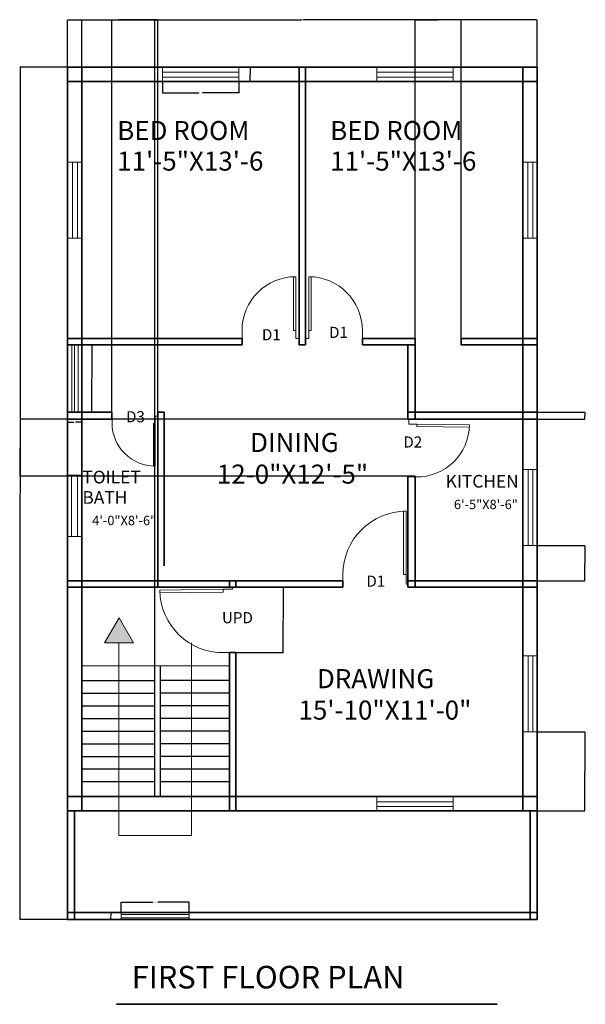
# Model space of a CAD drawing. Units: inches. Extents: x 2000 to 5103, y 1720 to 4295.
# Tile 2 of 2: x 2539 to 2895, y 1750 to 2371. Entities that reach past the tile are written whole.
import ezdxf

# ---------------------------------------------------------------- set-up
doc = ezdxf.new("R2010")
doc.units = ezdxf.units.IN
for name, color, linetype, lineweight in [('A-ANNO-DIMS', 2, 'Continuous', 18), ('A-ANNO-SYMB', 7, 'Continuous', 18), ('A-ANNO-TEXT', 3, 'Continuous', 18), ('A-ANNO-TITL', 7, 'Continuous', 35), ('A-AREA-IDEN', 7, 'Continuous', 25), ('A-DOOR', 4, 'Continuous', 18), ('A-WALL', 7, 'Continuous', 35), ('stair', 7, 'Continuous', 25), ('window', 10, 'Continuous', 18)]:
    doc.layers.add(name, color=color, linetype=linetype, lineweight=lineweight)
doc.styles.get("Standard").update_dxf_attribs({"font": 'arial.ttf'})
doc.dimstyles.get("Standard").update_dxf_attribs({"dimtxt": 0.18, "dimasz": 0.18, "dimexe": 0.18, "dimexo": 0.0625, "dimgap": 0.09, "dimtad": 0, "dimtih": 1, "dimtoh": 1, "dimdec": 4, "dimzin": 0, "dimdsep": 46, "dimtxsty": 'Standard', "dimcen": 0.09, "dimadec": 0, "dimazin": 0, "dimtfac": 1, "dimtdec": 4, "dimtofl": 0, "dimtmove": 0, "dimatfit": 3, "dimfxl": 1, "dimtolj": 1, "dimtzin": 0, "dimarcsym": 0})

# ---------------------------------------------------------------- blocks, each defined once
blk = doc.blocks.new('Dining Set - 36 x 72 in')
at = {"layer": 'window'}
for p, q in [((418.4, 887.02), (466.4, 887.02)), ((418.4, 883.92), (466.4, 883.92))]:
    blk.add_line(p, q, dxfattribs=at)
blk.add_lwpolyline([(418.4, 881.14), (418.4, 890.14), (466.4, 890.14), (466.4, 881.14)], close=True, dxfattribs=at)
blk = doc.blocks.new('*U3')
for p, q in [((0, 0), (0, -6)), ((40, 0), (40, -6))]:
    blk.add_line(p, q)
blk.add_lwpolyline([(0, 0), (0, 40), (1.75, 40), (1.75, 0)], close=True)
blk.add_arc((0, 0), 40, 0, 90)
blk = doc.blocks.new('WIN-DINING')
for p, q in [((2.68, 42.5), (2.68, 0)), ((4.5, 42.5), (4.5, 0)), ((6.78, 42.5), (6.78, 0))]:
    blk.add_line(p, q)
blk.add_lwpolyline([(0, 42.5), (9, 42.5), (9, 0), (0, 0)], close=True)
blk = doc.blocks.new('WIN-BATH')
for p, q in [((2.49, 38.59), (2.49, 0)), ((6.38, 38.59), (6.38, 0)), ((6.38, 38.59), (6.38, 0))]:
    blk.add_line(p, q)
blk.add_lwpolyline([(0, 38.59), (9, 38.59), (9, 0), (0, 0)], close=True)
blk = doc.blocks.new('WIN-FRONT')
for p, q in [((0, 3.25), (43.02, 3.25)), ((0, 1.25), (43.02, 1.25))]:
    blk.add_line(p, q)
blk.add_lwpolyline([(0, 4.5), (43.02, 4.5), (43.02, 0), (0, 0)], close=True)
blk = doc.blocks.new('STAIR-RETURN-FLIGHTS')
for p, q in [((93.06, 82.39), (0, 82.3)), ((46.1, 0), (46.1, 82.34)), ((49.5, 82.35), (49.5, 0)), ((0, 73.28), (46.1, 73.28)), ((49.5, 73.48), (93.06, 73.48)), ((0, 65.3), (46.1, 65.3)), ((49.5, 65.5), (93.06, 65.5)), ((0, 57.32), (46.1, 57.32)), ((49.5, 57.52), (93.06, 57.52)), ((0, 49.34), (46.1, 49.34)), ((49.5, 49.54), (93.06, 49.54)), ((0, 41.37), (46.1, 41.37)), ((49.5, 41.56), (93.06, 41.56)), ((0, 33.39), (46.1, 33.39)), ((49.5, 33.58), (93.06, 33.58)), ((0, 25.41), (46.1, 25.41)), ((49.5, 25.61), (93.06, 25.61)), ((0, 17.43), (46.1, 17.43)), ((49.5, 17.63), (93.06, 17.63)), ((0, 9.45), (46.1, 9.45)), ((49.5, 9.65), (93.06, 9.65))]:
    blk.add_line(p, q)
blk = doc.blocks.new('STAIR-PATH-ARROW')
h = blk.add_hatch(color=256)
h.dxf.hatch_style = 1
h.paths.add_polyline_path([(9.07, 137.14), (0, 121.43), (18.13, 121.43)])
for p, q in [((0, 121.43), (9.07, 137.14)), ((9.07, 137.14), (18.13, 121.43)), ((18.13, 121.43), (0, 121.43)), ((8.84, 0), (8.84, 121.43)), ((8.84, 121.43), (18.13, 121.43)), ((54.71, 121.43), (54.71, 0)), ((54.71, 0), (8.84, 0))]:
    blk.add_line(p, q)
blk = doc.blocks.new('*D9')
at = {"layer": 'A-ANNO-DIMS', "color": 0, "lineweight": -2, "transparency": 16777216}
for p, q in [((2629.1, 2331.91), (2629.1, 2324.59)), ((2677.1, 2331.91), (2677.1, 2324.59)), ((2629.28, 2324.77), (2651.98, 2324.77)), ((2676.92, 2324.77), (2654.22, 2324.77))]:
    blk.add_line(p, q, dxfattribs=at)
at = {"layer": 'A-ANNO-DIMS', "color": 0, "transparency": 16777216}
for points in [[(2629.28, 2324.8), (2629.28, 2324.74), (2629.1, 2324.77)], [(2676.92, 2324.8), (2676.92, 2324.74), (2677.1, 2324.77)]]:
    blk.add_solid(points, dxfattribs=at)
at = {"layer": 'Defpoints', "color": 0, "transparency": 16777216}
for p in [(2629.1, 2331.97), (2677.1, 2331.97), (2677.1, 2324.77)]:
    blk.add_point(p, dxfattribs=at)
at = {"layer": 'A-ANNO-DIMS', "color": 0, "transparency": 16777216, "insert": (2653.1, 2324.77), "char_height": 0.18, "attachment_point": 5}
blk.add_mtext('\\A1;WINDOW 48 TYP.', dxfattribs=at)
blk = doc.blocks.new('*D10')
at = {"layer": 'A-ANNO-DIMS', "color": 0, "lineweight": -2, "transparency": 16777216}
for p, q in [((2677.16, 2340.97), (2684.48, 2340.97)), ((2684.3, 2340.79), (2684.3, 2336.65)), ((2684.3, 2332.15), (2684.3, 2336.29)), ((2677.16, 2331.97), (2684.48, 2331.97))]:
    blk.add_line(p, q, dxfattribs=at)
at = {"layer": 'A-ANNO-DIMS', "color": 0, "transparency": 16777216}
for points in [[(2684.27, 2340.79), (2684.33, 2340.79), (2684.3, 2340.97)], [(2684.27, 2332.15), (2684.33, 2332.15), (2684.3, 2331.97)]]:
    blk.add_solid(points, dxfattribs=at)
at = {"layer": 'Defpoints', "color": 0, "transparency": 16777216}
for p in [(2677.1, 2340.97), (2684.3, 2340.97), (2677.1, 2331.97)]:
    blk.add_point(p, dxfattribs=at)
at = {"layer": 'A-ANNO-DIMS', "color": 0, "transparency": 16777216, "insert": (2684.3, 2336.47), "char_height": 0.18, "attachment_point": 5}
blk.add_mtext('\\A1;9 TYP.', dxfattribs=at)
blk = doc.blocks.new('*D11')
at = {"layer": 'A-ANNO-DIMS', "color": 0, "lineweight": -2, "transparency": 16777216}
for p, q in [((2578.24, 2165.97), (2584.74, 2165.97)), ((2584.56, 2165.79), (2584.56, 2144.9)), ((2584.56, 2123.65), (2584.56, 2144.54)), ((2578.24, 2123.47), (2584.74, 2123.47))]:
    blk.add_line(p, q, dxfattribs=at)
at = {"layer": 'A-ANNO-DIMS', "color": 0, "transparency": 16777216}
for points in [[(2584.53, 2165.79), (2584.59, 2165.79), (2584.56, 2165.97)], [(2584.53, 2123.65), (2584.59, 2123.65), (2584.56, 2123.47)]]:
    blk.add_solid(points, dxfattribs=at)
at = {"layer": 'Defpoints', "color": 0, "transparency": 16777216}
for p in [(2578.18, 2165.97), (2584.56, 2165.97), (2578.18, 2123.47)]:
    blk.add_point(p, dxfattribs=at)
at = {"layer": 'A-ANNO-DIMS', "color": 0, "transparency": 16777216, "insert": (2584.56, 2144.72), "char_height": 0.18, "attachment_point": 5}
blk.add_mtext('\\A1;WINDOW 43 TYP.', dxfattribs=at)
blk = doc.blocks.new('*D12')
at = {"layer": 'A-ANNO-DIMS', "color": 0, "lineweight": -2, "transparency": 16777216}
for p, q in [((2569.18, 2123.41), (2569.18, 2116.91)), ((2578.18, 2123.41), (2578.18, 2116.91)), ((2569.36, 2117.09), (2573.22, 2117.09)), ((2578, 2117.09), (2574.14, 2117.09))]:
    blk.add_line(p, q, dxfattribs=at)
at = {"layer": 'A-ANNO-DIMS', "color": 0, "transparency": 16777216}
for points in [[(2569.36, 2117.12), (2569.36, 2117.06), (2569.18, 2117.09)], [(2578, 2117.12), (2578, 2117.06), (2578.18, 2117.09)]]:
    blk.add_solid(points, dxfattribs=at)
at = {"layer": 'Defpoints', "color": 0, "transparency": 16777216}
for p in [(2569.18, 2123.47), (2578.18, 2123.47), (2578.18, 2117.09)]:
    blk.add_point(p, dxfattribs=at)
at = {"layer": 'A-ANNO-DIMS', "color": 0, "transparency": 16777216, "insert": (2573.68, 2117.09), "char_height": 0.18, "attachment_point": 5}
blk.add_mtext('\\A1;9 TYP.', dxfattribs=at)
blk = doc.blocks.new('*D15')
at = {"layer": 'A-ANNO-DIMS', "color": 0, "lineweight": -2, "transparency": 16777216}
for p, q in [((2602.94, 1807.94), (2602.94, 1814.51)), ((2603.12, 1814.33), (2622.88, 1814.33)), ((2645.78, 1814.33), (2626.03, 1814.33)), ((2645.96, 1807.94), (2645.96, 1814.51))]:
    blk.add_line(p, q, dxfattribs=at)
at = {"layer": 'A-ANNO-DIMS', "color": 0, "transparency": 16777216}
for points in [[(2603.12, 1814.36), (2603.12, 1814.3), (2602.94, 1814.33)], [(2645.78, 1814.36), (2645.78, 1814.3), (2645.96, 1814.33)]]:
    blk.add_solid(points, dxfattribs=at)
at = {"layer": 'Defpoints', "color": 0, "transparency": 16777216}
for p in [(2645.96, 1814.33), (2602.94, 1807.88), (2645.96, 1807.88)]:
    blk.add_point(p, dxfattribs=at)
at = {"layer": 'A-ANNO-DIMS', "color": 0, "transparency": 16777216, "insert": (2624.45, 1814.33), "char_height": 0.18, "attachment_point": 5}
blk.add_mtext('\\A1;FRONT WINDOW 43 TYP.', dxfattribs=at)
blk = doc.blocks.new('*D16')
at = {"layer": 'A-ANNO-DIMS', "color": 0, "lineweight": -2, "transparency": 16777216}
for p, q in [((2602.88, 1807.88), (2596.31, 1807.88)), ((2596.49, 1807.7), (2596.49, 1805.81)), ((2602.88, 1803.38), (2596.31, 1803.38)), ((2596.49, 1803.56), (2596.49, 1805.45))]:
    blk.add_line(p, q, dxfattribs=at)
at = {"layer": 'A-ANNO-DIMS', "color": 0, "transparency": 16777216}
for points in [[(2596.46, 1807.7), (2596.52, 1807.7), (2596.49, 1807.88)], [(2596.46, 1803.56), (2596.52, 1803.56), (2596.49, 1803.38)]]:
    blk.add_solid(points, dxfattribs=at)
at = {"layer": 'Defpoints', "color": 0, "transparency": 16777216}
for p in [(2596.49, 1807.88), (2602.94, 1807.88), (2602.94, 1803.38)]:
    blk.add_point(p, dxfattribs=at)
at = {"layer": 'A-ANNO-DIMS', "color": 0, "transparency": 16777216, "insert": (2596.49, 1805.63), "char_height": 0.18, "attachment_point": 5}
blk.add_mtext('\\A1;5 TYP.', dxfattribs=at)
blk = doc.blocks.new('*D21')
at = {"layer": 'A-ANNO-DIMS', "color": 0, "lineweight": -2, "transparency": 16777216}
for p, q in [((2569.18, 2341.03), (2569.18, 2370.95)), ((2569.36, 2370.77), (2716.89, 2370.77)), ((2865, 2370.77), (2717.47, 2370.77)), ((2865.18, 2341.03), (2865.18, 2370.95))]:
    blk.add_line(p, q, dxfattribs=at)
at = {"layer": 'A-ANNO-DIMS', "color": 0, "transparency": 16777216}
for points in [[(2569.36, 2370.8), (2569.36, 2370.74), (2569.18, 2370.77)], [(2865, 2370.8), (2865, 2370.74), (2865.18, 2370.77)]]:
    blk.add_solid(points, dxfattribs=at)
at = {"layer": 'Defpoints', "color": 0, "transparency": 16777216}
for p in [(2865.18, 2370.77), (2569.18, 2340.97), (2865.18, 2340.97)]:
    blk.add_point(p, dxfattribs=at)
at = {"layer": 'A-ANNO-DIMS', "color": 0, "transparency": 16777216, "insert": (2717.18, 2370.77), "char_height": 0.18, "attachment_point": 5}
blk.add_mtext('\\A1;296', dxfattribs=at)
blk = doc.blocks.new('*D22')
at = {"layer": 'A-ANNO-DIMS', "color": 0, "lineweight": -2, "transparency": 16777216}
for p, q in [((2569.12, 2340.97), (2539.2, 2340.97)), ((2539.38, 2340.79), (2539.38, 2072.36)), ((2539.38, 1803.56), (2539.38, 2071.99)), ((2569.12, 1803.38), (2539.2, 1803.38))]:
    blk.add_line(p, q, dxfattribs=at)
at = {"layer": 'A-ANNO-DIMS', "color": 0, "transparency": 16777216}
for points in [[(2539.35, 2340.79), (2539.41, 2340.79), (2539.38, 2340.97)], [(2539.35, 1803.56), (2539.41, 1803.56), (2539.38, 1803.38)]]:
    blk.add_solid(points, dxfattribs=at)
at = {"layer": 'Defpoints', "color": 0, "transparency": 16777216}
for p in [(2539.38, 2340.97), (2569.18, 2340.97), (2569.18, 1803.38)]:
    blk.add_point(p, dxfattribs=at)
at = {"layer": 'A-ANNO-DIMS', "color": 0, "transparency": 16777216, "insert": (2539.38, 2072.17), "char_height": 0.18, "attachment_point": 5}
blk.add_mtext('\\A1;537.6', dxfattribs=at)
blk = doc.blocks.new('*D29')
at = {"layer": 'A-ANNO-DIMS', "color": 0, "lineweight": -2, "transparency": 16777216}
for p, q in [((2865.36, 2039.26), (2895.28, 2039.26)), ((2895.1, 2039.08), (2895.1, 2028.29)), ((2895.1, 2017.15), (2895.1, 2027.93)), ((2865.24, 2016.97), (2895.28, 2016.97))]:
    blk.add_line(p, q, dxfattribs=at)
at = {"layer": 'A-ANNO-DIMS', "color": 0, "transparency": 16777216}
for points in [[(2895.07, 2039.08), (2895.13, 2039.08), (2895.1, 2039.26)], [(2895.07, 2017.15), (2895.13, 2017.15), (2895.1, 2016.97)]]:
    blk.add_solid(points, dxfattribs=at)
at = {"layer": 'Defpoints', "color": 0, "transparency": 16777216}
for p in [(2865.3, 2039.26), (2865.18, 2016.97), (2895.1, 2016.97)]:
    blk.add_point(p, dxfattribs=at)
at = {"layer": 'A-ANNO-DIMS', "color": 0, "transparency": 16777216, "insert": (2895.1, 2028.11), "char_height": 0.18, "attachment_point": 5}
blk.add_mtext('\\A1;22.287', dxfattribs=at)
blk = doc.blocks.new('*D30')
at = {"layer": 'A-ANNO-DIMS', "color": 0, "lineweight": -2, "transparency": 16777216}
for p, q in [((2865.36, 1921.87), (2895.28, 1921.87)), ((2895.1, 1921.69), (2895.1, 1897.1)), ((2895.1, 1872.15), (2895.1, 1896.74)), ((2865.24, 1871.97), (2895.28, 1871.97))]:
    blk.add_line(p, q, dxfattribs=at)
at = {"layer": 'A-ANNO-DIMS', "color": 0, "transparency": 16777216}
for points in [[(2895.07, 1921.69), (2895.13, 1921.69), (2895.1, 1921.87)], [(2895.07, 1872.15), (2895.13, 1872.15), (2895.1, 1871.97)]]:
    blk.add_solid(points, dxfattribs=at)
at = {"layer": 'Defpoints', "color": 0, "transparency": 16777216}
for p in [(2865.3, 1921.87), (2865.18, 1871.97), (2895.1, 1871.97)]:
    blk.add_point(p, dxfattribs=at)
at = {"layer": 'A-ANNO-DIMS', "color": 0, "transparency": 16777216, "insert": (2895.1, 1896.92), "char_height": 0.18, "attachment_point": 5}
blk.add_mtext('\\A1;49.9', dxfattribs=at)
blk = doc.blocks.new('*D32')
at = {"layer": 'A-ANNO-DIMS', "color": 0, "lineweight": -2, "transparency": 16777216}
for p, q in [((2597.18, 2123.53), (2597.18, 2370.95)), ((2597.36, 2370.77), (2611.46, 2370.77)), ((2626, 2370.77), (2611.9, 2370.77)), ((2626.18, 2123.53), (2626.18, 2370.95))]:
    blk.add_line(p, q, dxfattribs=at)
at = {"layer": 'A-ANNO-DIMS', "color": 0, "transparency": 16777216}
for points in [[(2597.36, 2370.8), (2597.36, 2370.74), (2597.18, 2370.77)], [(2626, 2370.8), (2626, 2370.74), (2626.18, 2370.77)]]:
    blk.add_solid(points, dxfattribs=at)
at = {"layer": 'Defpoints', "color": 0, "transparency": 16777216}
for p in [(2626.18, 2370.77), (2597.18, 2123.47), (2626.18, 2123.47)]:
    blk.add_point(p, dxfattribs=at)
at = {"layer": 'A-ANNO-DIMS', "color": 0, "transparency": 16777216, "insert": (2611.68, 2370.77), "char_height": 0.18, "attachment_point": 5}
blk.add_mtext('\\A1;29', dxfattribs=at)
blk = doc.blocks.new('*D33')
at = {"layer": 'A-ANNO-DIMS', "color": 0, "lineweight": -2, "transparency": 16777216}
for p, q in [((2783.62, 2118.97), (2539.2, 2118.97)), ((2539.38, 2118.79), (2539.38, 2101.15)), ((2539.38, 2083.15), (2539.38, 2100.79)), ((2783.62, 2082.97), (2539.2, 2082.97))]:
    blk.add_line(p, q, dxfattribs=at)
at = {"layer": 'A-ANNO-DIMS', "color": 0, "transparency": 16777216}
for points in [[(2539.35, 2118.79), (2539.41, 2118.79), (2539.38, 2118.97)], [(2539.35, 2083.15), (2539.41, 2083.15), (2539.38, 2082.97)]]:
    blk.add_solid(points, dxfattribs=at)
at = {"layer": 'Defpoints', "color": 0, "transparency": 16777216}
for p in [(2783.68, 2118.97), (2539.38, 2082.97), (2783.68, 2082.97)]:
    blk.add_point(p, dxfattribs=at)
at = {"layer": 'A-ANNO-DIMS', "color": 0, "transparency": 16777216, "insert": (2539.38, 2100.97), "char_height": 0.18, "attachment_point": 5}
blk.add_mtext('\\A1;36', dxfattribs=at)
blk = doc.blocks.new('*D36')
at = {"layer": 'A-ANNO-DIMS', "color": 0, "lineweight": -2, "transparency": 16777216}
for p, q in [((2675.3, 2012.97), (2705.22, 2012.97)), ((2705.04, 2012.79), (2705.04, 1992.65)), ((2705.04, 1972.15), (2705.04, 1992.29)), ((2675.3, 1971.97), (2705.22, 1971.97))]:
    blk.add_line(p, q, dxfattribs=at)
at = {"layer": 'A-ANNO-DIMS', "color": 0, "transparency": 16777216}
for points in [[(2705.01, 2012.79), (2705.07, 2012.79), (2705.04, 2012.97)], [(2705.01, 1972.15), (2705.07, 1972.15), (2705.04, 1971.97)]]:
    blk.add_solid(points, dxfattribs=at)
at = {"layer": 'Defpoints', "color": 0, "transparency": 16777216}
for p in [(2675.24, 2012.97), (2675.24, 1971.97), (2705.04, 1971.97)]:
    blk.add_point(p, dxfattribs=at)
at = {"layer": 'A-ANNO-DIMS', "color": 0, "transparency": 16777216, "insert": (2705.04, 1992.47), "char_height": 0.18, "attachment_point": 5}
blk.add_mtext('\\A1;41', dxfattribs=at)
blk = doc.blocks.new('*D37')
at = {"layer": 'A-ANNO-DIMS', "color": 0, "lineweight": -2, "transparency": 16777216}
for p, q in [((2788.18, 2166.03), (2788.18, 2370.95)), ((2788.36, 2370.77), (2802.46, 2370.77)), ((2817, 2370.77), (2802.9, 2370.77)), ((2817.18, 2166.03), (2817.18, 2370.95))]:
    blk.add_line(p, q, dxfattribs=at)
at = {"layer": 'A-ANNO-DIMS', "color": 0, "transparency": 16777216}
for points in [[(2788.36, 2370.8), (2788.36, 2370.74), (2788.18, 2370.77)], [(2817, 2370.8), (2817, 2370.74), (2817.18, 2370.77)]]:
    blk.add_solid(points, dxfattribs=at)
at = {"layer": 'Defpoints', "color": 0, "transparency": 16777216}
for p in [(2817.18, 2370.77), (2788.18, 2165.97), (2817.18, 2165.97)]:
    blk.add_point(p, dxfattribs=at)
at = {"layer": 'A-ANNO-DIMS', "color": 0, "transparency": 16777216, "insert": (2802.68, 2370.77), "char_height": 0.18, "attachment_point": 5}
blk.add_mtext('\\A1;29', dxfattribs=at)
blk = doc.blocks.new('*D39')
at = {"layer": 'A-ANNO-DIMS', "color": 0, "lineweight": -2, "transparency": 16777216}
for p, q in [((2865.24, 2123.47), (2895.28, 2123.47)), ((2865.24, 2118.97), (2895.28, 2118.97)), ((2895.1, 2123.29), (2895.1, 2121.4)), ((2895.1, 2119.15), (2895.1, 2121.04))]:
    blk.add_line(p, q, dxfattribs=at)
at = {"layer": 'A-ANNO-DIMS', "color": 0, "transparency": 16777216}
for points in [[(2895.07, 2123.29), (2895.13, 2123.29), (2895.1, 2123.47)], [(2895.07, 2119.15), (2895.13, 2119.15), (2895.1, 2118.97)]]:
    blk.add_solid(points, dxfattribs=at)
at = {"layer": 'Defpoints', "color": 0, "transparency": 16777216}
for p in [(2865.18, 2123.47), (2865.18, 2118.97), (2895.1, 2118.97)]:
    blk.add_point(p, dxfattribs=at)
at = {"layer": 'A-ANNO-DIMS', "color": 0, "transparency": 16777216, "insert": (2895.1, 2121.22), "char_height": 0.18, "attachment_point": 5}
blk.add_mtext('\\A1;4.5', dxfattribs=at)
blk = doc.blocks.new('*D40')
at = {"layer": 'A-ANNO-DIMS', "color": 0, "lineweight": -2, "transparency": 16777216}
for p, q in [((2578.18, 1963.33), (2578.18, 2370.95)), ((2578.36, 2370.77), (2600.92, 2370.77)), ((2624.1, 2370.77), (2601.54, 2370.77)), ((2624.28, 1963.38), (2624.28, 2370.95))]:
    blk.add_line(p, q, dxfattribs=at)
at = {"layer": 'A-ANNO-DIMS', "color": 0, "transparency": 16777216}
for points in [[(2578.36, 2370.8), (2578.36, 2370.74), (2578.18, 2370.77)], [(2624.1, 2370.8), (2624.1, 2370.74), (2624.28, 2370.77)]]:
    blk.add_solid(points, dxfattribs=at)
at = {"layer": 'Defpoints', "color": 0, "transparency": 16777216}
for p in [(2624.28, 2370.77), (2578.18, 1963.27), (2624.28, 1963.31)]:
    blk.add_point(p, dxfattribs=at)
at = {"layer": 'A-ANNO-DIMS', "color": 0, "transparency": 16777216, "insert": (2601.23, 2370.77), "char_height": 0.18, "attachment_point": 5}
blk.add_mtext('\\A1;46.1', dxfattribs=at)

msp = doc.modelspace()

# ---------------------------------------------------------------- linework, layer by layer
at = {"layer": 'A-ANNO-TITL'}
msp.add_line((2600, 1750), (2840, 1750), dxfattribs=at)
at = {"layer": 'A-DOOR'}
for p, q in [((2713.0045, 2169.9682), (2715.1814, 2169.9682)), ((2721.1694, 2169.9682), (2719.1814, 2169.9682)), ((2624.6103, 2121.0108), (2626.1814, 2121.0108)), ((2784.2595, 2115.9195), (2784.2595, 2118.9682)), ((2673.242, 2011.8135), (2673.242, 2012.9682)), ((2782.6495, 2014.9682), (2783.6814, 2014.9682))]:
    msp.add_line(p, q, dxfattribs=at)
at = {"layer": 'A-WALL'}
for p, q in [((2569.1814, 2340.9682), (2569.1814, 1871.9682)), ((2569.1814, 2340.9682), (2865.1814, 2340.9682)), ((2578.1814, 2340.9682), (2578.1814, 1871.9682)), ((2715.1814, 2340.9682), (2715.1814, 2165.9682)), ((2719.1814, 2340.9682), (2719.1814, 2165.9682)), ((2856.1814, 2340.9682), (2856.1814, 1871.9682)), ((2865.1814, 2340.9682), (2865.1814, 1871.9682)), ((2569.1814, 2331.9682), (2865.1814, 2331.9682)), ((2569.1814, 2169.9682), (2679.1814, 2169.9682)), ((2679.1814, 2165.9682), (2679.1814, 2169.9682)), ((2755.1814, 2165.9682), (2755.1814, 2169.9682)), ((2755.1814, 2169.9682), (2788.1814, 2169.9682)), ((2788.1814, 2169.9682), (2788.1814, 2118.9682)), ((2817.1814, 2165.9682), (2817.1814, 2169.9682)), ((2817.1814, 2169.9682), (2865.1814, 2169.9682)), ((2569.1814, 2165.9682), (2679.1814, 2165.9682)), ((2715.1814, 2165.9682), (2719.1814, 2165.9682)), ((2755.1814, 2165.9682), (2788.1814, 2165.9682)), ((2783.6814, 2165.9682), (2783.6814, 2118.9682)), ((2817.1814, 2165.9682), (2865.1814, 2165.9682)), ((2569.1814, 2123.4682), (2597.1814, 2123.4682)), ((2569.1814, 2118.9682), (2597.1814, 2118.9682)), ((2597.1814, 2118.9682), (2597.1814, 2123.4682)), ((2626.1814, 2123.4682), (2626.1814, 2012.9682)), ((2626.1814, 2123.4682), (2630.1081, 2123.4682)), ((2630.1081, 2123.4682), (2630.1081, 2026.4739)), ((2783.6814, 2123.4682), (2865.1814, 2123.4682)), ((2783.6814, 2118.9682), (2865.1814, 2118.9682)), ((2788.1814, 2082.9682), (2783.6814, 2082.9682)), ((2783.6814, 2082.9682), (2783.6814, 2012.9682)), ((2788.1814, 2082.9682), (2788.1814, 2012.9682)), ((2569.1814, 2016.9682), (2742.6814, 2016.9682)), ((2569.1814, 2012.9682), (2742.6814, 2012.9682)), ((2671.242, 2016.9682), (2671.242, 2012.9682)), ((2675.242, 2016.9682), (2675.242, 2012.9682)), ((2742.6814, 2012.9682), (2742.6814, 2016.9682)), ((2783.6814, 2016.9682), (2865.1814, 2016.9682)), ((2783.6814, 2012.9682), (2783.6814, 2012.9682)), ((2783.6814, 2012.9682), (2865.1814, 2012.9682)), ((2675.242, 1971.9682), (2671.242, 1971.9682)), ((2671.242, 1971.9682), (2671.242, 1871.9682)), ((2675.242, 1971.9682), (2675.242, 1871.9682)), ((2569.1814, 1880.9682), (2865.1814, 1880.9682)), ((2569.1814, 1871.9682), (2865.1814, 1871.9682)), ((2569.1814, 1871.9682), (2569.1814, 1803.3794)), ((2573.6814, 1871.9682), (2573.6814, 1803.3794)), ((2860.6814, 1803.3794), (2860.6814, 1871.9682)), ((2865.1814, 1803.3794), (2865.1814, 1871.9682)), ((2569.1814, 1807.8794), (2865.1814, 1807.8794)), ((2569.1814, 1803.3794), (2865.1814, 1803.3794))]:
    msp.add_line(p, q, dxfattribs=at)

# ---------------------------------------------------------------- block references
at = {"layer": 'A-ANNO-SYMB'}
msp.add_blockref('STAIR-PATH-ARROW', (2592.6023, 1856.5313), dxfattribs=at)
at = {"layer": 'A-DOOR'}
for p, xscale, yscale, zscale in [((2713.0045, 2175.0417), -0.8455769532508881, 0.8455769532508881, 0.8455769532508881), ((2721.1694, 2175.0417), 0.8455769532508881, 0.8455769532508881, 0.8455769532508881), ((2782.6495, 2020.9634), -0.9992024495959569, 0.9992024495959569, 0.9992024495959569)]:
    msp.add_blockref('*U3', p, dxfattribs=dict(at, xscale=xscale, yscale=yscale, zscale=zscale))
for p, xscale, yscale, zscale, rotation in [((2624.5099, 2116.5837), 0.680435440491929, 0.680435440491929, 0.680435440491929, 180), ((2789.247, 2115.8473), 0.8313368246920212, 0.8313368246920212, 0.8313368246920212, 269.1712141329585), ((2667.2474, 2011.7268), -0.9992024495959569, 0.9992024495959569, 0.9992024495959569, 90.82878586703616)]:
    msp.add_blockref('*U3', p, dxfattribs=dict(at, xscale=xscale, yscale=yscale, zscale=zscale, rotation=rotation))
at = {"layer": 'stair'}
msp.add_blockref('STAIR-RETURN-FLIGHTS', (2578.1814, 1880.9682), dxfattribs=at)
at = {"layer": 'window'}
for name, p in [('Dining Set - 36 x 72 in', (2210.6979, 1450.8296)), ('Dining Set - 36 x 72 in', (2345.7771, 1450.8296)), ('WIN-DINING', (2569.1814, 2123.4682)), ('WIN-BATH', (2569.1814, 2045.0502)), ('Dining Set - 36 x 72 in', (2345.7771, 990.7352)), ('WIN-FRONT', (2602.9411, 1803.3794))]:
    msp.add_blockref(name, p, dxfattribs=at)
at = {"layer": 'window', "rotation": 90}
for p in [(3459.32, 1814.7007), (3746.3105, 1814.7007), (3746.4388, 1620.8507), (3746.4388, 1503.464)]:
    msp.add_blockref('Dining Set - 36 x 72 in', p, dxfattribs=at)

# ---------------------------------------------------------------- texts
at = {"layer": 'A-ANNO-DIMS'}
for s, height, p in [('11\'-5"X13\'-6', 12, (2600.5056, 2275.772)), ('11\'-5"X13\'-6', 12, (2734.7098, 2275.772)), ('12-0"X12\'-5"', 12, (2663.315, 2078.3657)), ('6\'-5"X8\'-6"', 5.914719, (2812.6962, 2062.2832)), ('4\'-0"X8\'-6"', 5.914719, (2584.7801, 2052.1701)), ('15\'-10"X11\'-0"', 12, (2714.7507, 1929.5381))]:
    msp.add_text(s, height=height, dxfattribs=at).set_placement(p)
at = {"layer": 'A-ANNO-TEXT'}
for s, p in [('D1', (2691.7014, 2168.7704)), ('D1', (2734.016, 2170.262)), ('D3', (2606.0764, 2117.0622)), ('D2', (2780.8402, 2101.1102)), ('D1', (2757.5298, 2013.3804)), ('UPD', (2666.5243, 1990.3132))]:
    msp.add_text(s, height=7, dxfattribs=at).set_placement(p)
at = {"layer": 'A-ANNO-TITL'}
msp.add_text('FIRST FLOOR PLAN', height=14.242438, dxfattribs=at).set_placement((2609.6537, 1760))
at = {"layer": 'A-AREA-IDEN'}
for s, height, p in [('BED ROOM', 12, (2600.5056, 2295.0489)), ('BED ROOM', 12, (2734.7098, 2295.0489)), ('DINING', 12, (2684.2552, 2098.3173)), ('TOILET', 8, (2578.6097, 2078.4882)), ('KITCHEN', 8, (2807.4758, 2075.8458)), ('BATH', 8, (2578.6097, 2065.6369)), ('DRAWING', 12, (2726.3678, 1949.3675))]:
    msp.add_text(s, height=height, dxfattribs=at).set_placement(p)

# ---------------------------------------------------------------- dimensions: what is measured, and where the dimension line sits
at = {"layer": 'A-ANNO-DIMS'}
for base, p1, p2, override, picture, middle in [((2865.1814, 2370.7682), (2569.1814, 2340.9682), (2865.1814, 2340.9682), {"dimdec": 0, "dimlfac": 1, "dimrnd": 0, "dimzin": 0, "dimdsep": 46, "dimlunit": 2}, '*D21', (2717.1814, 2370.7682)), ((2624.2841, 2370.7682), (2578.1814, 1963.2679), (2624.2841, 1963.313), {"dimdec": 1, "dimlfac": 1, "dimrnd": 0, "dimzin": 0, "dimdsep": 46, "dimlunit": 2}, '*D40', (2601.2328, 2370.7682)), ((2626.1814, 2370.7682), (2597.1814, 2123.4682), (2626.1814, 2123.4682), {"dimdec": 0, "dimlfac": 1, "dimrnd": 0, "dimzin": 0, "dimdsep": 46, "dimlunit": 2}, '*D32', (2611.6814, 2370.7682)), ((2817.1814, 2370.7682), (2788.1814, 2165.9682), (2817.1814, 2165.9682), {"dimdec": 0, "dimlfac": 1, "dimrnd": 0, "dimzin": 0, "dimdsep": 46, "dimlunit": 2}, '*D37', (2802.6814, 2370.7682))]:
    dim = msp.add_linear_dim(base=base, p1=p1, p2=p2, dimstyle='Standard', override=override, dxfattribs=at)
    dim.commit()
    dim.dimension.update_dxf_attribs({"geometry": picture, "text_midpoint": middle})
for base, p1, p2, angle, override, picture, middle in [((2539.3814, 2340.9682), (2569.1814, 1803.3794), (2569.1814, 2340.9682), 90, {"dimdec": 1, "dimlfac": 1, "dimrnd": 0, "dimzin": 0, "dimdsep": 46, "dimlunit": 2}, '*D22', (2539.3814, 2072.1738)), ((2539.3814, 2082.9682), (2783.6814, 2118.9682), (2783.6814, 2082.9682), 90, {"dimdec": 0, "dimlfac": 1, "dimrnd": 0, "dimzin": 0, "dimdsep": 46, "dimlunit": 2}, '*D33', (2539.3814, 2100.9682)), ((2895.1002, 2118.9682), (2865.1814, 2123.4682), (2865.1814, 2118.9682), 90, {"dimdec": 1, "dimlfac": 1, "dimrnd": 0, "dimzin": 0, "dimdsep": 46, "dimlunit": 2}, '*D39', (2895.1002, 2121.2182)), ((2895.1002, 2016.9682), (2865.3002, 2039.255), (2865.1814, 2016.9682), 90, {"dimdec": 3, "dimlfac": 1, "dimrnd": 0, "dimzin": 0, "dimdsep": 46, "dimlunit": 2}, '*D29', (2895.1002, 2028.1116)), ((2705.042, 1971.9682), (2675.242, 2012.9682), (2675.242, 1971.9682), 270, {"dimdec": 0, "dimlfac": 1, "dimrnd": 0, "dimzin": 0, "dimdsep": 46, "dimlunit": 2}, '*D36', (2705.042, 1992.4682)), ((2895.1002, 1871.9682), (2865.3002, 1921.8683), (2865.1814, 1871.9682), 90, {"dimdec": 1, "dimlfac": 1, "dimrnd": 0, "dimzin": 0, "dimdsep": 46, "dimlunit": 2}, '*D30', (2895.1002, 1896.9182))]:
    dim = msp.add_linear_dim(base=base, p1=p1, p2=p2, angle=angle, dimstyle='Standard', override=override, dxfattribs=at)
    dim.commit()
    dim.dimension.update_dxf_attribs({"geometry": picture, "text_midpoint": middle})
for base, p1, p2, text, picture, middle in [((2684.3022, 2340.9682), (2677.1022, 2331.9682), (2677.1022, 2340.9682), '<> TYP.', '*D10', (2684.3022, 2336.4682)), ((2584.5564161834, 2165.9681952973), (2578.1814161834, 2123.4681952973), (2578.1814161834, 2165.9681952973), 'WINDOW <> TYP.', '*D11', (2584.5564161834, 2144.7181952973)), ((2596.4875341946, 1807.8794345844), (2602.9410891211, 1803.3794345844), (2602.9410891211, 1807.8794345844), '<> TYP.', '*D16', (2596.4875341946, 1805.6294345844))]:
    dim = msp.add_linear_dim(base=base, p1=p1, p2=p2, angle=90, text=text, dimstyle='Standard', override={"dimdec": 0, "dimlfac": 1, "dimrnd": 0, "dimzin": 0, "dimdsep": 46, "dimlunit": 2}, dxfattribs=at)
    dim.commit()
    dim.dimension.update_dxf_attribs({"geometry": picture, "text_midpoint": middle})
for base, p1, p2, text, picture, middle in [((2677.1022, 2324.7682), (2629.1022, 2331.9682), (2677.1022, 2331.9682), 'WINDOW <> TYP.', '*D9', (2653.1022, 2324.7682)), ((2578.1814, 2117.0932), (2569.1814, 2123.4682), (2578.1814, 2123.4682), '<> TYP.', '*D12', (2573.6814, 2117.0932)), ((2645.9648, 1814.333), (2602.9411, 1807.8794), (2645.9648, 1807.8794), 'FRONT WINDOW <> TYP.', '*D15', (2624.4529, 1814.333))]:
    dim = msp.add_linear_dim(base=base, p1=p1, p2=p2, text=text, dimstyle='Standard', override={"dimdec": 0, "dimlfac": 1, "dimrnd": 0, "dimzin": 0, "dimdsep": 46, "dimlunit": 2}, dxfattribs=at)
    dim.commit()
    dim.dimension.update_dxf_attribs({"geometry": picture, "text_midpoint": middle})

doc.saveas('drawing.dxf')
